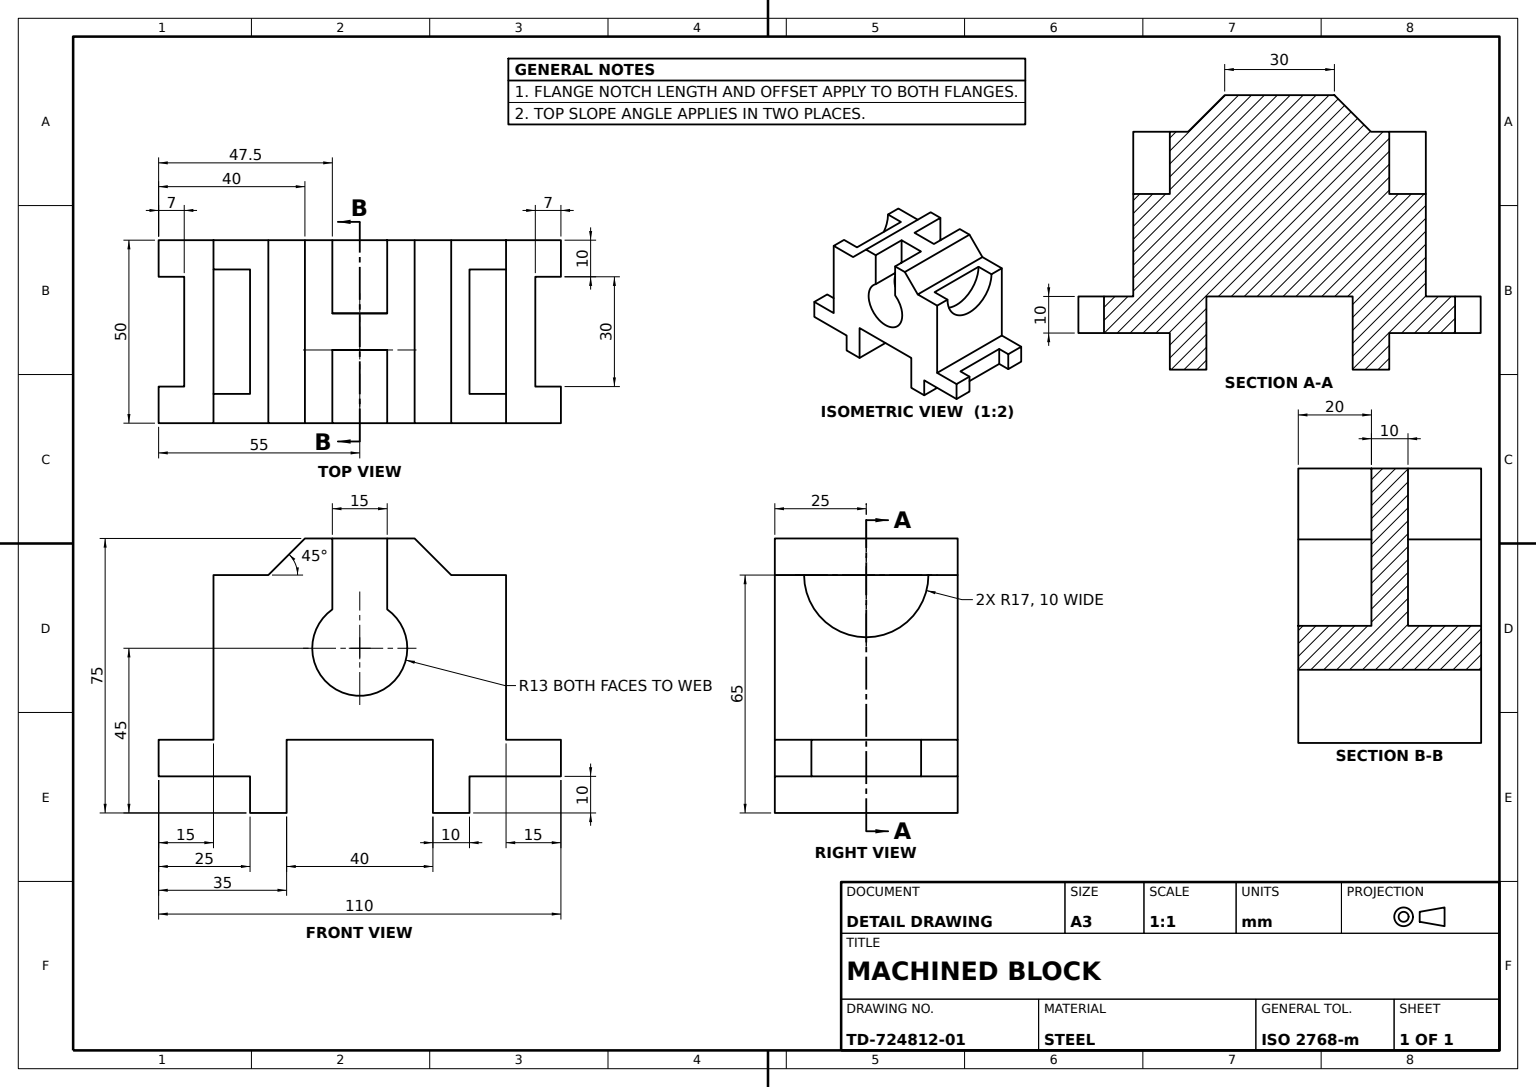
SolidWorks part; units mm, degrees
material "Plain Carbon Steel"
ref_plane "Front Plane" through (0, 0, 0) normal (0, 0, 1) x (1, 0, 0)
ref_plane "Top Plane" through (0, 0, 0) normal (0, 1, 0) x (1, 0, 0)
ref_plane "Right Plane" through (0, 0, 0) normal (1, 0, 0) x (0, 0, -1)
sketch "Base Body Profile Sketch" plane through (0, 0, 0) normal (0, 0, 1) x (1, 0, 0)
  line L0 (0, 0) -> (25, 0)
  line L1 (25, 0) -> (25, -10)
  line L2 (25, -10) -> (35, -10)
  line L3 (35, -10) -> (35, 10)
  line L4 (35, 10) -> (75, 10)
  line L5 (75, 10) -> (75, -10)
  line L6 (75, -10) -> (85, -10)
  line L7 (85, -10) -> (85, 0)
  line L8 (85, 0) -> (110, 0)
  line L9 (110, 0) -> (110, 10)
  line L14 (62.5, 48) -> (62.5, 45.6184)
  line L15 (47.5, 65) -> (47.5, 48)
  line L16 (47.5, 48) -> (47.5, 45.6184)
  line L18 (62.5, 48) -> (62.5, 65)
  line L22 (15, 10) -> (15, 55)
  line L23 (15, 10) -> (0, 10)
  line L24 (0, 10) -> (0, 0)
  line L25 (110, 10) -> (95, 10)
  line L26 (95, 10) -> (95, 55)
  line L27 (15, 55) -> (30, 55)
  line L28 (95, 55) -> (80, 55)
  line L29 (47.5, 65) -> (40, 65)
  line L30 (40, 65) -> (30, 55)
  line L31 (62.5, 65) -> (70, 65)
  line L32 (70, 65) -> (80, 55)
  arc A0 (47.5, 45.6184) -> (62.5, 45.6184) centre (55, 35) ccw
  point P12 (110, 5)
  dimension "D1" = 26
  dimension "D8" = 13
  dimension "D2" = 15
  dimension "D3" = 45
  dimension "D4" = 65
  dimension "D5" = 75
  dimension "D6" = 55
  dimension "D7" = 40
  dimension "D9" = 15
  dimension "D10" = 15
  dimension "D11" = 20
  dimension "D12" = 25
  dimension "D13" = 10
  dimension "D14" = 10
  dimension "D15" = 110
  dimension "D16" = 15
  dimension "D17" = 17
  dimension "D18" = 35
extrude "Base Body" add sketch "Base Body Profile Sketch" along normal blind 50
sketch "Upper Block Sketch" plane through (0, 65, 0) normal (0, 1, 0) x (1, 0, 0)
  line L0 (47.5, -25) -> (47.5, -20)
  line L1 (47.5, -50) -> (47.5, 0) construction
  line L2 (47.5, -20) -> (47.5, -30)
  line L3 (47.5, -50) -> (47.5, 0) construction
  line L4 (47.5, -30) -> (62.5, -30)
  line L5 (62.5, -50) -> (62.5, 0) construction
  line L6 (62.5, -30) -> (62.5, -20)
  line L7 (62.5, -50) -> (62.5, 0) construction
  line L8 (62.5, -20) -> (47.5, -20)
  line L9 (70, 0) -> (62.5, 0) construction
  line M2 (62.5, 0) -> (62.5, -50)
  dimension "D1" = 20
extrude "Upper Block" add sketch "Upper Block Sketch" against normal blind 50 contours L8 L0 L2 L4 M2
sketch "Centre Web Sketch" plane through (0, 0, 30) normal (0, 0, 1) x (1, 0, 0)
  line L0 (47.5, 45.6184) -> (47.5, 24.3816)
  line L1 (62.5, 45.6184) -> (62.5, 24.3816)
  arc A0 (47.5, 45.6184) -> (47.5, 24.3816) centre (55, 35) ccw
  arc A1 (62.5, 24.3816) -> (62.5, 45.6184) centre (55, 35) ccw
  dimension "D1" = 26
extrude "Centre Web" add sketch "Centre Web Sketch" against normal blind 10
sketch "Foot Slot 1 Sketch" plane through (0, 0, 0) normal (-1, 0, 0) x (0, 0, 1)
  line L0 (25, 10) -> (10, 10)
  line L1 (50, 10) -> (0, 10) construction
  line L2 (10, 10) -> (10, 0)
  line L3 (50, 0) -> (0, 0) construction
  line L4 (10, 0) -> (40, 0)
  line L5 (50, 0) -> (0, 0) construction
  line L6 (40, 0) -> (40, 10)
  line L7 (50, 10) -> (0, 10) construction
  line L8 (40, 10) -> (25, 10)
  dimension "D1" = 10
extrude "Foot Slot 1" cut sketch "Foot Slot 1 Sketch" against normal blind 7
sketch "Foot Slot 2 Sketch" plane through (110, 0, 0) normal (1, 0, 0) x (0, 0, -1)
  line L0 (-25, 10) -> (-40, 10)
  line L1 (-50, 10) -> (0, 10) construction
  line L2 (-40, 10) -> (-40, 0)
  line L3 (-50, 0) -> (0, 0) construction
  line L4 (-40, 0) -> (-10, 0)
  line L5 (-50, 0) -> (0, 0) construction
  line L6 (-10, 0) -> (-10, 10)
  line L7 (-50, 10) -> (0, 10) construction
  line L8 (-10, 10) -> (-25, 10)
  line L9 (0, 0) -> (0, 10) construction
  dimension "D1" = 10
extrude "Foot Slot 2" cut sketch "Foot Slot 2 Sketch" against normal blind 7
sketch "Bearing Seat Cut 1 Sketch" plane through (95, 0, 0) normal (1, 0, 0) x (0, 0, -1)
  line L0 (-50, 55) -> (0, 55) construction
  line L1 (-42, 55) -> (-8, 55)
  arc A0 (-42, 55) -> (-8, 55) centre (-25, 55) ccw
  dimension "D1" = 17
extrude "Bearing Seat Cut 1" cut sketch "Bearing Seat Cut 1 Sketch" against normal blind 10
sketch "Bearing Seat Cut 2 Sketch" plane through (15, 0, 0) normal (-1, 0, 0) x (0, 0, 1)
  line L0 (50, 55) -> (0, 55) construction
  line L1 (8, 55) -> (42, 55)
  arc A0 (8, 55) -> (42, 55) centre (25, 55) ccw
  dimension "D1" = 17
extrude "Bearing Seat Cut 2" cut sketch "Bearing Seat Cut 2 Sketch" against normal blind 10
